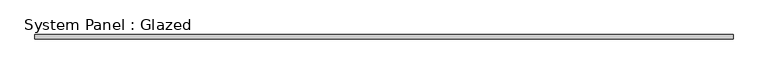
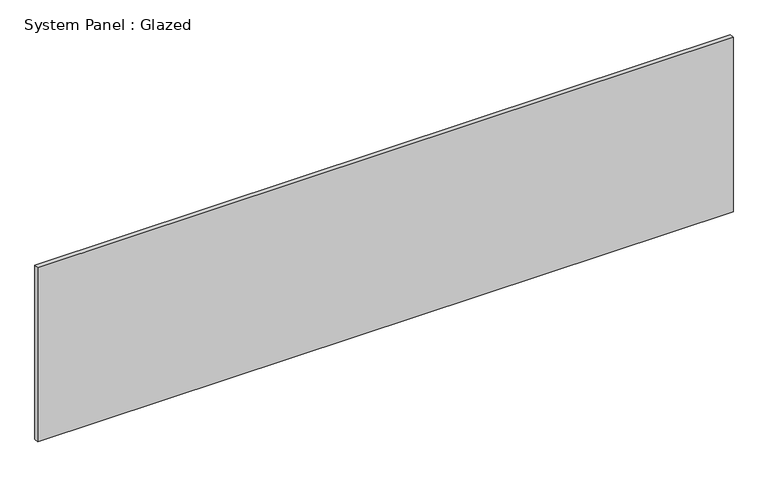
"""IFC4 building model written with IfcOpenShell, lengths in millimetres: plate geometry, System Panel : Glazed."""

from ifc_helpers import new_model, si_unit, origin, origin_with_axes, place, context, project, spatial, polyline, outline, extrude, source, transform, mapped, element, save


def system_panel_glazed_f04aca20(model_context):
    return source(origin(), model_context, "Body", "SweptSolid", [
        extrude(outline(polyline([(1955.8, 19.05), (-1955.8, 19.05), (-1955.8, 44.45), (1955.8, 44.45), (1955.8, 19.05)])), origin_with_axes(), (0.0, 0.0, 1.0), 1035.1943025),
    ])


if __name__ == "__main__":
    model = new_model("IFC4")
    model_context = context("Model", 3, world=origin())
    ifc_project = project(units=[si_unit("LENGTHUNIT", "METRE", prefix="MILLI")], contexts=[model_context])
    site = spatial("IfcSite", under=ifc_project)
    building = spatial("IfcBuilding", under=site)
    placement = place(None, origin())
    system_panel_glazed_shape = system_panel_glazed_f04aca20(model_context)
    element("IfcPlate", 1, ObjectType="System Panel : Glazed", at=placement, inside=building, context=model_context, shape_type="MappedRepresentation", body=[
        mapped(system_panel_glazed_shape, transform((0.0, 0.0, 0.0), x_axis=(1.0, 0.0, 0.0), y_axis=(0.0, 1.0, 0.0), z_axis=(0.0, 0.0, 1.0))),
    ])
    save(model, "model.ifc")

# Revit data of these elements
# Type "System Panel : Glazed"
#   Construction Type Id = "GSP4R"
#   Analytic Construction = "1/8 in Pilkington single glazing"
#   Visual Light Transmittance = 0.9
#   Solar Heat Gain Coefficient = 0.86
#   Heat Transfer Coefficient (U) = 1.18115 BTU/(h·ft²·°F)
#   Define Thermal Properties by = 1
# Element 1 (IfcPlate, "System Panel : Glazed")
#   Materials on its faces: "Glass"
# Materials
#   "Glass": class "Glass", colour RGB 0 128 192, transparency 0.75, Description = "Soda Lime Glass", Cost = 0
